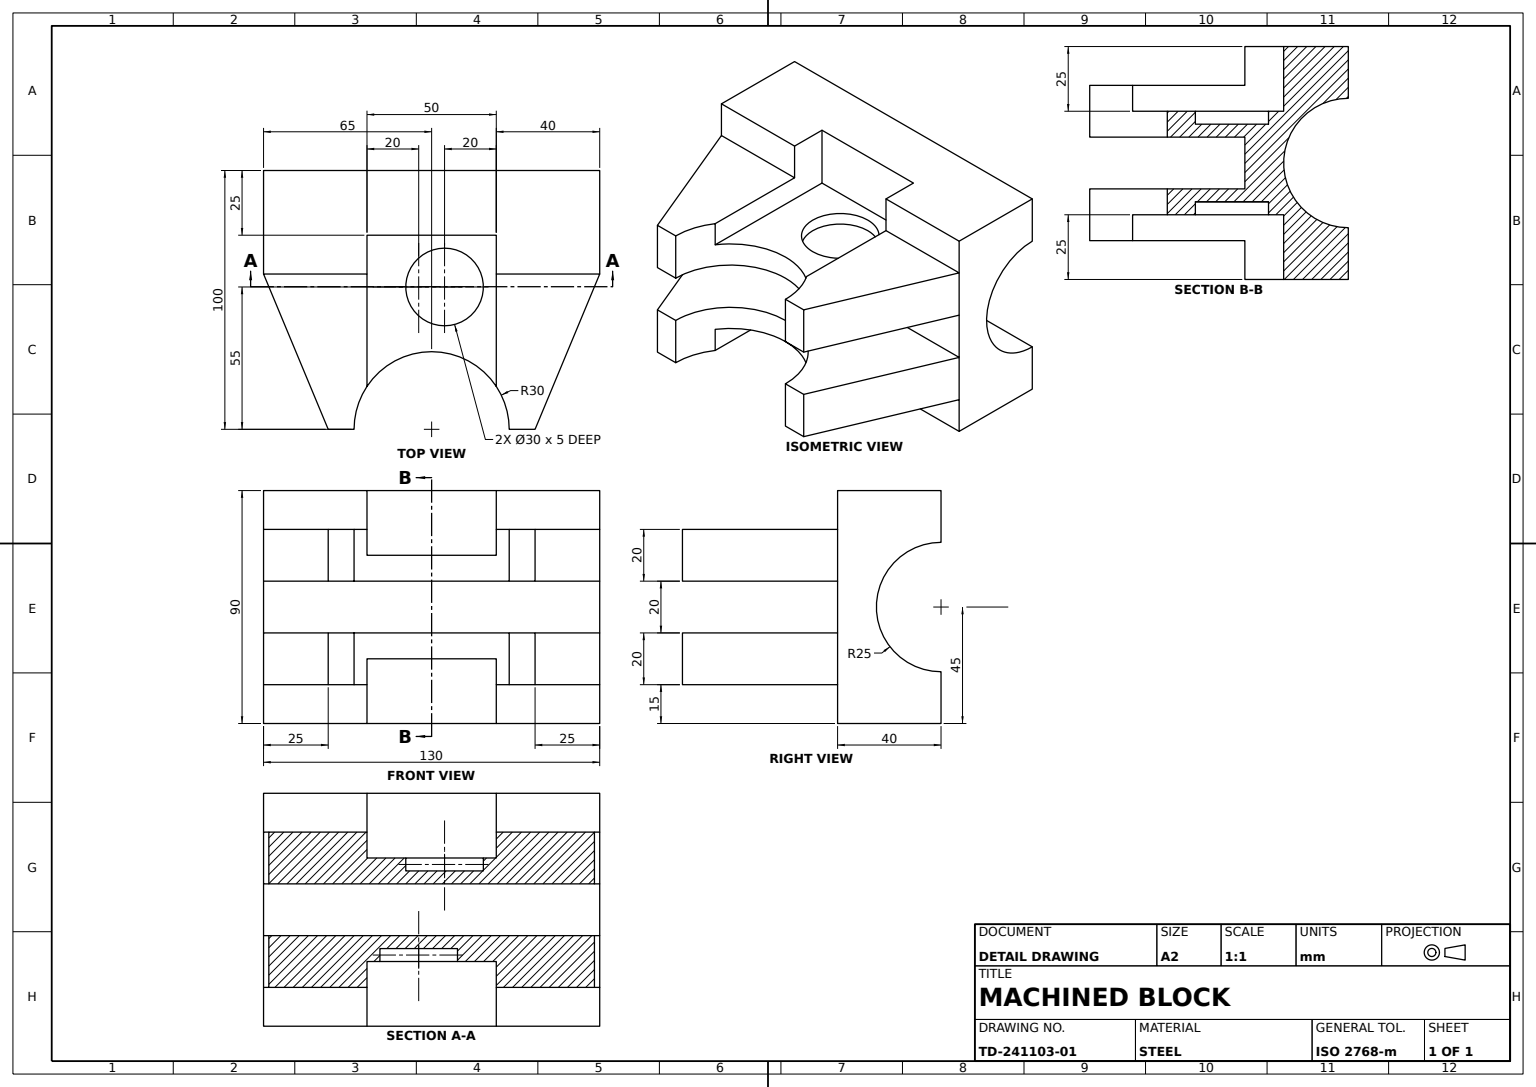
from build123d import *
from build123d.topology import SkipClean

# Parameters (mm, degrees)
BASE_BLOCK_SKETCH_W             = 130
BASE_BLOCK_SKETCH_H             = 90
BASE_BLOCK_40_DEPTH             = 40
SIDE_POCKET_A_25_DEPTH          = 25
SIDE_POCKET_B_25_DEPTH          = 25
UPPER_BOSS_50_DEPTH             = 50
WEB_BOSS_10_DEPTH               = 10
WEB_NOTCH_A_10_DEPTH            = 10
WEB_NOTCH_B_10_DEPTH            = 10
SLOT_CUT_A_60_DEPTH             = 60
SLOT_START                      = -60
SLOT_CUT_B_60_DEPTH             = 60
SLOT_CUT_C_60_DEPTH             = 60
SPOT_FACE_A_SKETCH_R            = 15
SPOT_FACE_A_30X5_DEPTH          = 5
SPOT_FACE_B_SKETCH_R            = 15
SPOT_FACE_B_30X5_DEPTH          = 5
BEARING_CRADLE_50_THROUGH_DEPTH = 130


with BuildPart() as part:
    # Base Block Sketch → Base Block 40 (new body)
    with BuildSketch(Plane.XY):
        with Locations((65, 45)):
            Rectangle(BASE_BLOCK_SKETCH_W, BASE_BLOCK_SKETCH_H)
    extrude(amount=BASE_BLOCK_40_DEPTH)

    # Side Pocket A Sketch → Side Pocket A 25 (cut)
    with BuildSketch(Plane.XZ):
        Polygon((65, 40), (40, 40), (40, 25), (90, 25), (90, 40), align=None)
    extrude(amount=-SIDE_POCKET_A_25_DEPTH, mode=Mode.SUBTRACT)

    # Side Pocket B Sketch → Side Pocket B 25 (cut)
    with BuildSketch(Plane(origin=(0, 90, 0), x_dir=(1, 0, 0), z_dir=(0, 1, 0))):
        Polygon((65, -40), (90, -40), (90, -25), (40, -25), (40, -40), align=None)
    extrude(amount=-SIDE_POCKET_B_25_DEPTH, mode=Mode.SUBTRACT)

    # Upper Boss Sketch → Upper Boss 50 (add)
    with BuildSketch(Plane.XZ.offset(-25)):
        Polygon((65, 100), (105, 100), (130, 40), (0, 40), (25, 100), align=None)
    extrude(amount=-UPPER_BOSS_50_DEPTH)

    # Web Boss Sketch → Web Boss 10 (add)
    with BuildSketch(Plane.XZ.offset(-25)):
        Polygon((0, 40), (25, 100), (105, 100), (130, 40), (90, 40), (40, 40), align=None)
    extrude(amount=WEB_BOSS_10_DEPTH)

    # Web Notch A Sketch → Web Notch A 10 (cut)
    with BuildSketch(Plane.XZ.offset(-15)):
        with BuildLine():
            Line((90, 100), (40, 100))
            ThreePointArc((40, 100), (65, 75), (90, 100))
        make_face()
        with BuildLine():
            ThreePointArc((40, 100), (65, 75), (90, 100))
            Line((90, 100), (90, 40))
            Line((90, 40), (40, 40))
            Line((40, 40), (40, 100))
        make_face()
    extrude(amount=-WEB_NOTCH_A_10_DEPTH, mode=Mode.SUBTRACT)

    # Web Notch B Sketch → Web Notch B 10 (cut)
    with BuildSketch(Plane(origin=(0, 75, 0), x_dir=(1, 0, 0), z_dir=(0, 1, 0))):
        with BuildLine():
            ThreePointArc((90, -100), (65, -75), (40, -100))
            Line((40, -100), (40, -40))
            Line((40, -40), (90, -40))
            Line((90, -40), (90, -100))
        make_face()
        with BuildLine():
            ThreePointArc((90, -100), (65, -75), (40, -100))
            Line((40, -100), (90, -100))
        make_face()
    extrude(amount=-WEB_NOTCH_B_10_DEPTH, mode=Mode.SUBTRACT)

    # Slot Cut A Sketch → Slot Cut A 60 (cut)
    with BuildSketch(Plane.XZ.offset(-25)):
        with BuildLine():
            Line((35, 100), (95, 100))
            ThreePointArc((95, 100), (65, 70), (35, 100))
        make_face()
    extrude(amount=-SLOT_CUT_A_60_DEPTH, mode=Mode.SUBTRACT)

    # Slot Cut B Sketch → Slot Cut B 60 (cut)
    with SkipClean():  # the faces are left unmerged after this step: merging them gives an invalid solid
        with BuildSketch(Plane(origin=(0, 25, 0), x_dir=(1, 0, 0), z_dir=(0, 1, 0)).offset(SLOT_START)):
            with BuildLine():
                Line((40, -100), (40, -83.416876048))
                ThreePointArc((40, -83.416876048), (36.277186767, -91.339745962), (35, -100))
                Line((35, -100), (40, -100))
            make_face()
            with BuildLine():
                Line((90, -100), (90, -83.416876048))
                ThreePointArc((90, -83.416876048), (93.722813233, -91.339745962), (95, -100))
                Line((95, -100), (90, -100))
            make_face()
        extrude(amount=SLOT_CUT_B_60_DEPTH, mode=Mode.SUBTRACT)

    # Slot Cut C Sketch → Slot Cut C 60 (cut)
    with SkipClean():  # the faces are left unmerged after this step: merging them gives an invalid solid
        with BuildSketch(Plane.XY.offset(100)):
            Polygon((25, 55), (105, 55), (130, 55), (130, 35), (0, 35), (0, 55), align=None)
        extrude(amount=-SLOT_CUT_C_60_DEPTH, mode=Mode.SUBTRACT)

    # Spot Face A Sketch → Spot Face A Ø30x5 (cut)
    with SkipClean():  # the faces are left unmerged after this step: merging them gives an invalid solid
        with BuildSketch(Plane.XZ.offset(-25)):
            with Locations(Location((60, 45, 0), (0, 0, 270))):
                Circle(SPOT_FACE_A_SKETCH_R)
        extrude(amount=-SPOT_FACE_A_30X5_DEPTH, mode=Mode.SUBTRACT)

    # Spot Face B Sketch → Spot Face B Ø30x5 (cut)
    with SkipClean():  # the faces are left unmerged after this step: merging them gives an invalid solid
        with BuildSketch(Plane(origin=(0, 65, 0), x_dir=(1, 0, 0), z_dir=(0, 1, 0))):
            with Locations(Location((70, -45, 0), (0, 0, 270))):
                Circle(SPOT_FACE_B_SKETCH_R)
        extrude(amount=-SPOT_FACE_B_30X5_DEPTH, mode=Mode.SUBTRACT)

    # Bearing Cradle Sketch → Bearing Cradle Ø50 Through (cut)
    with SkipClean():  # the faces are left unmerged after this step: merging them gives an invalid solid
        with BuildSketch(Plane(origin=(130, 0, 0), x_dir=(0, 0, -1), z_dir=(1, 0, 0))):
            with BuildLine():
                Line((0, 70), (0, 20))
                ThreePointArc((0, 20), (-25, 45), (0, 70))
            make_face()
        extrude(amount=-BEARING_CRADLE_50_THROUGH_DEPTH, mode=Mode.SUBTRACT)


solid = part.part
